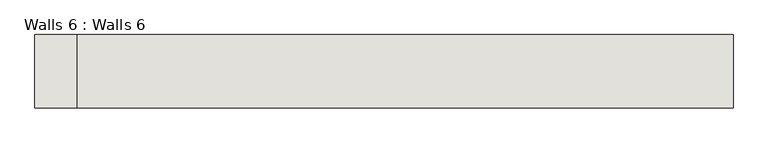
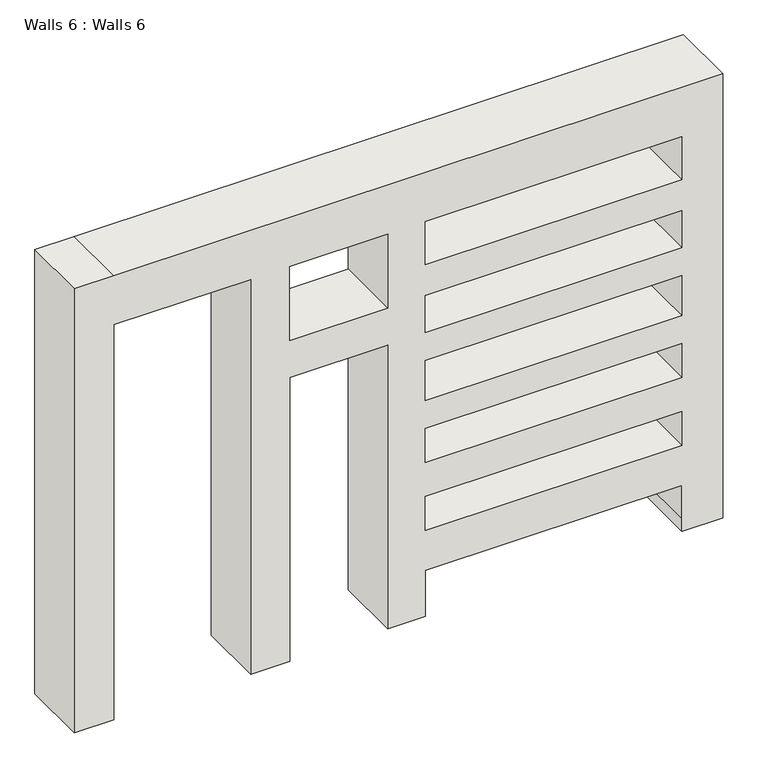
"""IFC4 building model written with IfcOpenShell, lengths in millimetres: wall geometry, Walls 6 : Walls 6."""

from ifc_helpers import new_model, si_unit, frame, origin, place, context, project, spatial, polyline, outline, extrude, source, transform, mapped, element, save


def walls_6_walls_6_78742a1b(model_context):
    return source(origin(), model_context, "Body", "SweptSolid", [
        extrude(outline(polyline([(3657.6, -9746.1043381), (3657.6, -10053.3997472), (0.0, -10053.3997472), (0.0, -9746.1043381), (3251.2, -9746.1043381), (3251.2, -8679.3043381), (0.0, -8679.3043381), (0.0, -8374.5043381), (2336.8, -8374.5043381), (2336.8, -7612.5043381), (0.0, -7612.5043381), (0.0, -7320.0927523), (101.6, -7320.0927523), (379.5257577, -7320.0927523), (379.5257577, -5322.0947327), (101.6, -5322.0947327), (0.0, -5322.0947327), (0.0, -5005.1497472), (3251.2, -5005.1497472), (3657.6, -5005.1497472), (3657.6, -9746.1043381)]), holes=[polyline([(2641.6, -7612.5043381), (2641.6, -8374.5043381), (3251.2, -8374.5043381), (3251.2, -7612.5043381), (2641.6, -7612.5043381)]), polyline([(3251.2, -5322.0947327), (2895.6, -5322.0947327), (2895.6, -7320.0927523), (3251.2, -7320.0927523), (3251.2, -5322.0947327)]), polyline([(2641.6, -5322.0947327), (2336.8, -5322.0947327), (2336.8, -7320.0927523), (2641.6, -7320.0927523), (2641.6, -5322.0947327)]), polyline([(2106.7257577, -5322.0947327), (1776.5257577, -5322.0947327), (1776.5257577, -7320.0927523), (2106.7257577, -7320.0927523), (2106.7257577, -5322.0947327)]), polyline([(1547.9257577, -5322.0947327), (1268.5257577, -5322.0947327), (1268.5257577, -7320.0927523), (1547.9257577, -7320.0927523), (1547.9257577, -5322.0947327)]), polyline([(989.1257577, -5322.0947327), (709.7257577, -5322.0947327), (709.7257577, -7320.0927523), (989.1257577, -7320.0927523), (989.1257577, -5322.0947327)])]), frame((0.0, 1153.7384838, 0.0), z_axis=(0.0, 1.0, 0.0), x_axis=(0.0, 0.0, 1.0)), (0.0, 0.0, 1.0), 528.5099644),
    ])


if __name__ == "__main__":
    model = new_model("IFC4")
    model_context = context("Model", 3, world=origin())
    ifc_project = project(units=[si_unit("LENGTHUNIT", "METRE", prefix="MILLI")], contexts=[model_context])
    site = spatial("IfcSite", under=ifc_project)
    building = spatial("IfcBuilding", under=site)
    placement = place(None, origin())
    walls_6_walls_6_shape = walls_6_walls_6_78742a1b(model_context)
    element("IfcWall", 1, ObjectType="Walls 6 : Walls 6", at=placement, inside=building, context=model_context, shape_type="MappedRepresentation", body=[
        mapped(walls_6_walls_6_shape, transform((0.0, 0.0, 0.0), x_axis=(1.0, 0.0, 0.0), y_axis=(0.0, 1.0, 0.0), z_axis=(0.0, 0.0, 1.0))),
    ])
    save(model, "model.ifc")

# Revit data of these elements
# Element 1 (IfcWall, "Walls 6 : Walls 6")
#   Materials on its faces: "Default Wall"
# Materials
#   "Default Wall": colour RGB 128 128 128, transparency 0
